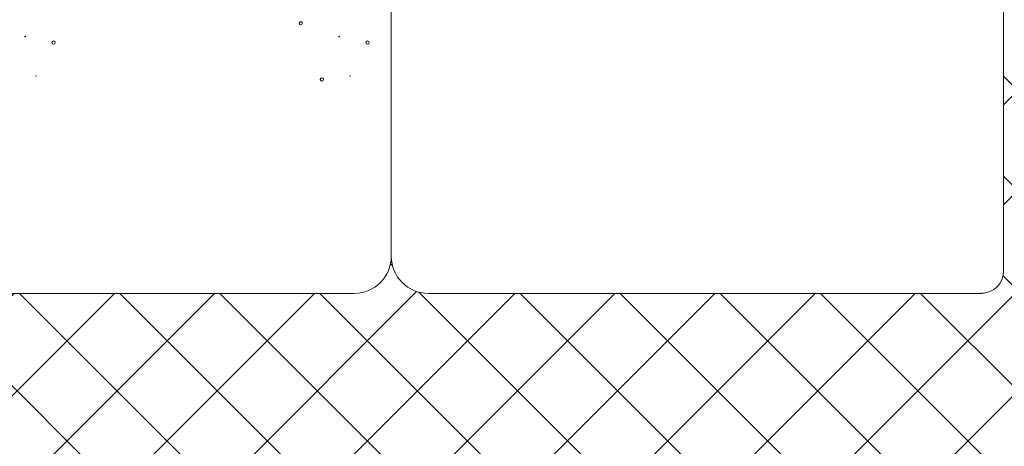
# Model space of a CAD drawing. Units: inches. Extents: x -466983 to 1020, y 324 to 318697.
# Tile 67 of 97: x 644 to 679, y 924 to 939. Entities that reach past the tile are written whole.
import ezdxf

# ---------------------------------------------------------------- set-up
doc = ezdxf.new("R2010")
doc.units = ezdxf.units.IN
doc.header["$MEASUREMENT"] = 0
doc.layers.add('A-FLOR-PATT', color=252, linetype='Continuous', lineweight=13)
doc.layers.add('A-FURN', color=8, linetype='Continuous', lineweight=18)

# ---------------------------------------------------------------- blocks, each defined once
blk = doc.blocks.new('L Shaped Sofa')
at = {"ltscale": 2}
for p, q in [((2356.696, 767.567), (2377.232, 767.567)), ((2377.232, 767.567), (2392.324, 767.567)), ((2429.959, 767.567), (2397.1, 767.567)), ((2355.263, 760.482), (2355.263, 766.134)), ((2394.712, 747.255), (2394.712, 765.179)), ((2355.263, 760.482), (2355.263, 736.259))]:
    blk.add_line(p, q, dxfattribs=at)
for centre, radius, start, end in [((2356.696, 766.134), 1.433, 90, 180), ((2392.324, 765.179), 2.388, 0, 90), ((2397.1, 765.179), 2.388, 90, 180), ((2399.184, 753.788), 0.106, 90, 270), ((2399.184, 753.788), 0.106, 270, 90), ((2397.375, 753.562), 0.0177, 90, 270), ((2397.375, 753.562), 0.0177, 270, 90), ((2417.604, 753.562), 0.0177, 90, 270), ((2417.604, 753.562), 0.0177, 270, 90), ((2396.244, 751.412), 0.106, 90, 270), ((2396.244, 751.412), 0.106, 270, 90), ((2416.474, 751.412), 0.106, 90, 270), ((2416.474, 751.412), 0.106, 270, 90), ((2398.074, 751.018), 0.0177, 90, 270), ((2398.074, 751.018), 0.0177, 270, 90), ((2418.303, 751.018), 0.0177, 90, 270), ((2418.303, 751.018), 0.0177, 270, 90), ((2400.541, 750.168), 0.106, 90, 270), ((2400.541, 750.168), 0.106, 270, 90)]:
    blk.add_arc(centre, radius, start, end, dxfattribs=at)

msp = doc.modelspace()

# ---------------------------------------------------------------- hatches: boundary and pattern name
at = {"layer": 'A-FLOR-PATT', "transparency": 33554572}
h = msp.add_hatch(dxfattribs=at)
h.set_pattern_fill('ANSI37', color=256, scale=30)
h.set_pattern_definition([(45, (-1212.4137, -290.035), (-2.6516504, 2.6516504), []), (135, (-1212.4137, -290.035), (-2.6516504, -2.6516504), [])])
h.paths.add_polyline_path([(901.806, 1075.938), (900.614, 1075.938), (900.614, 1065.386), (899.391, 1065.386), (898.091, 1065.386), (892.836, 1058.71, -0.258377), (892.188, 1058.351), (879.985, 1058.351, -0.20177), (879.438, 1058.581), (874.081, 1065.386), (872.781, 1065.386), (871.558, 1065.386), (871.558, 1075.938), (813.806, 1075.938), (813.806, 1044.792), (832.395, 1044.792, -0.394795), (848.66, 1028.536), (848.66, 1009.938), (901.806, 1009.938), (901.806, 1015.938), (901.306, 1015.938), (871.306, 1015.938), (871.306, 1017.25), (871.334, 1017.25, -0.401453), (901.306, 1045.938), (901.806, 1045.938)])
edge = h.paths.add_edge_path(flags=16)
edge.add_line((847.773, 1068.949), (847.773, 1073.709))
edge.add_arc((849.227, 1073.709), 1.454, 90, 180, ccw=False)
edge.add_line((849.227, 1075.163), (864.492, 1075.163))
edge.add_arc((864.492, 1073.709), 1.454, 0, 90, ccw=False)
edge.add_line((865.946, 1073.709), (865.946, 1069.004))
edge.add_arc((832.645, 1068.976), 33.301, -20.6123, 0.0472, ccw=False)
edge.add_ellipse((856.859, 1058.48), major_axis=(0, 10.213), ratio=0.685919, start_angle=100.0088, end_angle=259.9912, ccw=False)
edge.add_arc((881.074, 1068.976), 33.301, 180.0472, 200.6123, ccw=False)
h.paths.add_polyline_path([(853.146, 1066.482), (853.146, 1066.453), (853.146, 1066.453, 0.433107), (852.917, 1066.685), (852.917, 1066.453), (853.146, 1066.453), (853.146, 1066.482), (853.088, 1066.612, 0.697939), (852.7, 1066.453), (852.7, 1066.453), (852.7, 1066.482), (852.917, 1067.001), (852.917, 1066.685, -0.396254)], flags=0)
h.paths.add_polyline_path([(861.019, 1066.482), (861.019, 1066.453), (861.019, 1066.453, 0.416404), (860.802, 1066.685), (860.802, 1066.453), (861.019, 1066.453), (861.019, 1066.482), (860.967, 1066.605, 0.713344), (860.573, 1066.453), (860.573, 1066.453), (860.573, 1066.482), (860.802, 1067.001), (860.802, 1066.685, -0.379973)], flags=0)
edge = h.paths.add_edge_path(flags=0)
edge.add_spline(control_points=[(861.13, 1065.785), (861.466, 1065.248), (861.613, 1065.016), (861.983, 1064.374), (862.192, 1063.944), (862.561, 1063.039), (862.721, 1062.563), (862.987, 1061.578), (863.092, 1061.069), (863.245, 1060.031), (863.293, 1059.503), (863.329, 1058.441), (863.318, 1057.908), (863.237, 1056.852), (863.166, 1056.329), (862.97, 1055.308), (862.843, 1054.81), (862.537, 1053.852), (862.357, 1053.393), (861.951, 1052.525), (861.725, 1052.117), (861.233, 1051.362), (860.967, 1051.016), (860.405, 1050.395), (860.108, 1050.12), (859.494, 1049.646), (859.176, 1049.448), (858.528, 1049.13), (858.197, 1049.011), (857.531, 1048.852), (857.196, 1048.812), (856.525, 1048.812), (856.189, 1048.852), (855.524, 1049.01), (855.193, 1049.129), (854.545, 1049.447), (854.227, 1049.645), (853.612, 1050.118), (853.316, 1050.393), (852.753, 1051.014), (852.487, 1051.36), (851.995, 1052.114), (851.769, 1052.523), (851.363, 1053.39), (851.183, 1053.85), (850.877, 1054.807), (850.75, 1055.305), (850.553, 1056.326), (850.483, 1056.849), (850.401, 1057.905), (850.39, 1058.438), (850.426, 1059.5), (850.473, 1060.028), (850.626, 1061.066), (850.732, 1061.575), (850.997, 1062.561), (851.157, 1063.036), (851.525, 1063.942), (851.734, 1064.371), (852.106, 1065.016), (852.254, 1065.25), (852.608, 1065.733)], knot_values=[3.915332, 3.915332, 3.915332, 3.915332, 4.013468, 4.013468, 4.175532, 4.175532, 4.337596, 4.337596, 4.49966, 4.49966, 4.661724, 4.661724, 4.823788, 4.823788, 4.985852, 4.985852, 5.147916, 5.147916, 5.30998, 5.30998, 5.472044, 5.472044, 5.634109, 5.634109, 5.796173, 5.796173, 5.958237, 5.958237, 6.120301, 6.120301, 6.282365, 6.282365, 6.444429, 6.444429, 6.606493, 6.606493, 6.768557, 6.768557, 6.930621, 6.930621, 7.092685, 7.092685, 7.254749, 7.254749, 7.416813, 7.416813, 7.578878, 7.578878, 7.740942, 7.740942, 7.903006, 7.903006, 8.06507, 8.06507, 8.227134, 8.227134, 8.389198, 8.389198, 8.551262, 8.551262, 8.65037, 8.65037, 8.65037, 8.65037], degree=3, periodic=0)
edge.add_line((852.642, 1065.785), (861.13, 1065.785))
edge = h.paths.add_edge_path(flags=0)
edge.add_ellipse((856.85, 1057.743), major_axis=(0, 7.792), ratio=0.687861, start_angle=0, end_angle=360)
h.paths.add_polyline_path([(848.863, 1069.389), (848.863, 1073.96, -0.414214), (849.954, 1075.051), (863.765, 1075.051, -0.414214), (864.856, 1073.96), (864.856, 1069.389, -0.388936), (864.524, 1069.027, -0.043561), (849.195, 1069.027, -0.388936)], flags=0)
h.paths.add_polyline_path([(853.101, 1068.112, -1), (852.677, 1068.112, -1)], flags=0)
edge = h.paths.add_edge_path(flags=0)
edge.add_ellipse((856.859, 1057.338), major_axis=(0, 2.207), ratio=0.657164, start_angle=0, end_angle=360)
h.paths.add_polyline_path([(861.041, 1068.112, -1), (860.618, 1068.112, -1)], flags=0)
edge = h.paths.add_edge_path()
edge.add_line((573.954, 1057.341), (573.954, 1075.938))
edge.add_line((573.954, 1075.938), (558.731, 1075.938))
edge.add_line((558.731, 1075.938), (558.731, 1065.386))
edge.add_line((558.731, 1065.386), (557.507, 1065.386))
edge.add_line((557.507, 1065.386), (556.207, 1065.386))
edge.add_line((556.207, 1065.386), (550.952, 1058.71))
edge.add_arc((550.304, 1059.116), 0.765, 270, 327.9483, ccw=False)
edge.add_line((550.304, 1058.351), (538.101, 1058.351))
edge.add_arc((538.101, 1059.116), 0.765, 224.3704, 270, ccw=False)
edge.add_line((537.555, 1058.581), (532.198, 1065.386))
edge.add_line((532.198, 1065.386), (530.898, 1065.386))
edge.add_line((530.898, 1065.386), (529.674, 1065.386))
edge.add_line((529.674, 1065.386), (529.674, 1075.938))
edge.add_line((529.674, 1075.938), (520.806, 1075.938))
edge.add_line((520.806, 1075.938), (520.806, 1045.938))
edge.add_line((520.806, 1045.938), (521.306, 1045.938))
edge.add_arc((521.306, 1015.938), 30, 2.5075, 90, ccw=False)
edge.add_line((551.277, 1017.25), (551.306, 1017.25))
edge.add_line((551.306, 1017.25), (551.306, 1015.938))
edge.add_line((551.306, 1015.938), (520.806, 1015.938))
edge.add_line((520.806, 1015.938), (520.806, 1009.938))
edge.add_line((520.806, 1009.938), (559.191, 1010.402))
edge.add_arc((559.191, 1011.856), 1.454, 180, 270, ccw=False)
edge.add_line((557.737, 1011.856), (557.737, 1016.561))
edge.add_arc((591.039, 1016.589), 33.301, 159.3877, 180.0472, ccw=False)
edge.add_ellipse((566.824, 1027.085), major_axis=(0, 10.213), ratio=0.685919, start_angle=280.0088, end_angle=439.9912, ccw=False)
edge.add_arc((542.609, 1016.589), 33.301, 0.0472, 20.6123, ccw=False)
edge.add_line((575.91, 1016.616), (575.91, 1011.856))
edge.add_arc((574.456, 1011.856), 1.454, -90, 0, ccw=False)
edge.add_line((574.456, 1010.402), (608.806, 1009.938))
edge.add_line((608.806, 1009.938), (608.806, 1041.086))
edge.add_line((608.806, 1041.086), (590.218, 1041.086))
edge.add_arc((590.775, 1057.907), 16.831, 181.9277, 268.1032, ccw=False)
edge = h.paths.add_edge_path()
edge.add_ellipse((494.244, 583.62), major_axis=(0, 10.213), ratio=0.685919, start_angle=280.0088, end_angle=439.9912, ccw=False)
edge.add_arc((470.03, 573.124), 33.301, 0.0472, 20.6123, ccw=False)
edge.add_line((503.331, 573.152), (503.331, 568.392))
edge.add_arc((501.877, 568.392), 1.454, -90, 0, ccw=False)
edge.add_line((501.877, 566.938), (539.806, 566.938))
edge.add_line((539.806, 566.938), (539.806, 572.938))
edge.add_line((539.806, 572.938), (539.306, 572.938))
edge.add_line((539.306, 572.938), (509.306, 572.938))
edge.add_line((509.306, 572.938), (509.306, 574.25))
edge.add_line((509.306, 574.25), (509.334, 574.25))
edge.add_arc((539.306, 572.938), 30, 90, 177.4925, ccw=False)
edge.add_line((539.306, 602.938), (539.806, 602.938))
edge.add_line((539.806, 602.938), (539.806, 626.938))
edge.add_line((539.806, 626.938), (531.772, 626.938))
edge.add_line((531.772, 626.938), (531.772, 616.386))
edge.add_line((531.772, 616.386), (530.548, 616.386))
edge.add_line((530.548, 616.386), (529.249, 616.386))
edge.add_line((529.249, 616.386), (523.711, 609.351))
edge.add_line((523.711, 609.351), (510.777, 609.351))
edge.add_line((510.777, 609.351), (505.239, 616.386))
edge.add_line((505.239, 616.386), (503.939, 616.386))
edge.add_line((503.939, 616.386), (502.715, 616.386))
edge.add_line((502.715, 616.386), (502.715, 626.938))
edge.add_line((502.715, 626.938), (481.698, 626.938))
edge.add_line((481.698, 626.938), (481.698, 610.995))
edge.add_arc((467.27, 611.473), 14.436, 271.9277, 358.1032, ccw=False)
edge.add_line((467.756, 597.045), (451.806, 597.045))
edge.add_line((451.806, 597.045), (451.806, 584.404))
edge.add_line((451.806, 584.404), (451.806, 566.938))
edge.add_line((451.806, 566.938), (486.612, 566.938))
edge.add_arc((486.612, 568.392), 1.454, 180, 270, ccw=False)
edge.add_line((485.158, 568.392), (485.158, 573.097))
edge.add_arc((518.459, 573.124), 33.301, 159.3877, 180.0472, ccw=False)
h.paths.add_polyline_path([(836.261, 1020.733), (879.89, 1020.733), (879.89, 1039.39), (836.261, 1039.39)], flags=25)
h.paths.add_polyline_path([(549.985, 1036.749), (593.614, 1036.749), (593.614, 1055.407), (549.985, 1055.407)], flags=24)
h.paths.add_polyline_path([(475.123, 595.596), (518.752, 595.596), (518.752, 614.253), (475.123, 614.253)], flags=24)
h = msp.add_hatch(dxfattribs=at)
h.set_pattern_fill('ANSI37', color=256, scale=20)
h.set_pattern_definition([(45, (-1212.4137, -290.035), (-1.767767, 1.767767), []), (135, (-1212.4137, -290.035), (-1.767767, -1.767767), [])])
h.paths.add_polyline_path([(809.806, 870.938), (809.806, 888.152), (806.998, 888.152), (802.662, 888.152), (789.383, 888.152), (786.285, 888.152, -0.414214), (785.499, 888.937), (785.499, 900.196), (785.499, 908.47, -0.414214), (786.808, 909.779, -0.414214), (785.499, 911.088), (785.499, 929.101, -0.414214), (786.808, 930.411, -0.414214), (785.499, 931.72), (785.499, 931.904, -0.414214), (784.19, 930.595), (766.722, 930.595, -0.412359), (765.413, 931.896, -0.413741), (764.115, 930.578), (744.578, 930.422, -0.416556), (743.786, 931.207), (743.786, 933.515), (742.215, 933.515), (742.215, 952.024, -0.001344), (743.786, 952.2), (743.786, 953.938), (678.592, 953.938), (678.592, 951.131), (678.592, 946.794), (678.592, 933.515), (678.592, 930.417, -0.414214), (677.806, 929.631), (666.548, 929.631), (658.274, 929.631, -0.414214), (656.965, 930.94, -0.414214), (655.656, 929.631), (637.642, 929.631, -0.414214), (636.333, 930.94, -0.414214), (635.024, 929.631), (634.839, 929.631, -0.414214), (636.149, 928.322), (636.149, 910.854, -0.412359), (634.848, 909.545, -0.413741), (636.165, 908.247), (636.321, 888.71, -0.416556), (635.536, 887.918), (633.228, 887.918), (633.228, 886.347), (614.719, 886.347, -0.001344), (614.544, 887.918), (612.806, 887.918), (612.806, 834.938), (612.806, 752.938), (612.806, 748.938), (612.806, 697.938), (654.806, 697.938), (654.806, 701.938), (715.806, 701.938), (715.806, 737.435), (774.292, 737.435), (774.292, 795.938), (809.806, 795.938)])
h.paths.add_polyline_path([(679.276, 849.576, 0.102523), (682.148, 849.261, -0.080461), (694.543, 849.773, -0.283899), (694.482, 849.008, 0.136605), (694.407, 848.81, -0.030441), (694.543, 846.893), (694.543, 842.62), (694.543, 838.347, -0.028219), (694.425, 836.568), (694.425, 836.568, 0.196187), (694.446, 836.271, -0.302897), (694.543, 835.467, -0.080461), (682.148, 835.979, 0.102523), (679.276, 835.664, -0.58611), (678.646, 836.017), (678.646, 849.223, -0.58611)], flags=16)
h.paths.add_polyline_path([(679.517, 848.651, 0.699597), (679.476, 848.634, 1.20716), (679.194, 848.742, 0.010621)], flags=0)
h.paths.add_polyline_path([(679.492, 836.561, -0.013798), (679.918, 836.659, -0.071703), (682.853, 837.143, -0.165743), (682.166, 839.101), (682.166, 842.609), (682.166, 846.06, -0.240616), (683.473, 848.677, -0.068263), (693.929, 849.008), (693.788, 848.708), (693.788, 849.023, 0.067332), (683.473, 848.677, 0.240616), (682.166, 846.06), (682.166, 842.609), (682.166, 839.101, 0.23459), (683.461, 836.551, 0.068093), (693.788, 836.195), (693.788, 836.51), (693.93, 836.21, -0.077215), (682.242, 836.782, 0.086627), (679.528, 836.57, -0.628402), (679.503, 836.573), (679.503, 836.607, 0.910458)], flags=0)
h.paths.add_polyline_path([(679.476, 848.636), (679.207, 848.647), (679.207, 836.572, 0.913566), (679.365, 836.586), (679.476, 836.582)], flags=0)
h.paths.add_polyline_path([(679.276, 829.86, 0.102523), (682.148, 829.546, -0.080461), (694.543, 830.057, -0.283899), (694.482, 829.293, 0.136605), (694.407, 829.095, -0.030441), (694.543, 827.178), (694.543, 822.904), (694.543, 818.631, -0.028219), (694.425, 816.853), (694.425, 816.853, 0.196187), (694.446, 816.556, -0.302897), (694.543, 815.752, -0.080461), (682.148, 816.263, 0.102523), (679.276, 815.949, -0.58611), (678.646, 816.302), (678.646, 829.507, -0.58611)], flags=16)
h.paths.add_polyline_path([(679.517, 828.936, 0.699597), (679.476, 828.919, 1.20716), (679.194, 829.027, 0.010621)], flags=0)
h.paths.add_polyline_path([(679.492, 816.846, -0.013798), (679.918, 816.944, -0.071703), (682.853, 817.428, -0.165743), (682.166, 819.385), (682.166, 822.894), (682.166, 826.345, -0.240616), (683.473, 828.961, -0.068263), (693.929, 829.293), (693.788, 828.993), (693.788, 829.308, 0.067332), (683.473, 828.961, 0.240616), (682.166, 826.345), (682.166, 822.894), (682.166, 819.385, 0.23459), (683.461, 816.836, 0.068093), (693.788, 816.48), (693.788, 816.795), (693.93, 816.495, -0.077215), (682.242, 817.066, 0.086627), (679.528, 816.855, -0.628402), (679.503, 816.858), (679.503, 816.892, 0.910458)], flags=0)
h.paths.add_polyline_path([(679.476, 828.921), (679.207, 828.932), (679.207, 816.857, 0.913566), (679.365, 816.871), (679.476, 816.867)], flags=0)
h.paths.add_polyline_path([(679.276, 810.145, 0.102523), (682.148, 809.83, -0.080461), (694.543, 810.342, -0.3023), (694.447, 809.539, 0.10023), (694.406, 809.388, -0.03057), (694.543, 807.462), (694.543, 803.189), (694.543, 798.916, -0.03057), (694.406, 796.991, 0.10023), (694.447, 796.839, -0.3023), (694.543, 796.036, -0.080461), (682.148, 796.548, 0.102523), (679.276, 796.233, -0.58611), (678.646, 796.586), (678.646, 809.792, -0.58611)], flags=16)
h.paths.add_polyline_path([(679.517, 809.242, 0.699597), (679.476, 809.224, 1.20716), (679.194, 809.332, 0.010621)], flags=0)
h.paths.add_polyline_path([(679.492, 797.151, -0.013798), (679.918, 797.25, -0.071703), (682.853, 797.734, -0.165743), (682.166, 799.691), (682.166, 803.2), (682.166, 806.65, -0.239349), (683.461, 809.258, -0.072465), (694.447, 809.541, 0.197932), (694.425, 809.241), (693.788, 809.299), (693.788, 809.614, 0.068093), (683.461, 809.258, 0.239349), (682.166, 806.65), (682.166, 803.2), (682.166, 799.691, 0.235854), (683.473, 797.132, 0.067332), (693.788, 796.786), (693.788, 797.101), (694.425, 797.159, 0.197932), (694.447, 796.859, -0.080419), (682.156, 797.379, 0.083867), (679.528, 797.16, -0.628402), (679.503, 797.164), (679.503, 797.197, 0.910458)], flags=0)
h.paths.add_polyline_path([(679.207, 809.237), (679.207, 797.162, 0.913566), (679.365, 797.176), (679.476, 797.173), (679.476, 809.227)], flags=0)
h.paths.add_polyline_path([(695.364, 853.299), (728.223, 853.299), (728.223, 771.152), (695.364, 771.152)], flags=16)
h.paths.add_polyline_path([(696.021, 852.642), (727.566, 852.642), (727.566, 771.809), (696.021, 771.809)], flags=0)
h.paths.add_polyline_path([(679.276, 788.787, 0.102523), (682.148, 788.472, -0.080461), (694.543, 788.984, -0.3023), (694.447, 788.181, 0.10023), (694.406, 788.03, -0.03057), (694.543, 786.104), (694.543, 781.831), (694.543, 777.558, -0.03057), (694.406, 775.632, 0.10023), (694.447, 775.481, -0.3023), (694.543, 774.678, -0.080461), (682.148, 775.19, 0.102523), (679.276, 774.875, -0.58611), (678.646, 775.228), (678.646, 788.434, -0.58611)], flags=16)
h.paths.add_polyline_path([(679.517, 787.883, 0.699597), (679.476, 787.866, 1.20716), (679.194, 787.974, 0.010621)], flags=0)
h.paths.add_polyline_path([(679.492, 775.793, -0.013798), (679.918, 775.891, -0.071703), (682.853, 776.375, -0.165743), (682.166, 778.333), (682.166, 781.841), (682.166, 785.292, -0.239349), (683.461, 787.899, -0.072465), (694.447, 788.182, 0.197932), (694.425, 787.882), (693.788, 787.94), (693.788, 788.255, 0.068093), (683.461, 787.899, 0.239349), (682.166, 785.292), (682.166, 781.841), (682.166, 778.333, 0.235854), (683.473, 775.774, 0.067332), (693.788, 775.428), (693.788, 775.742), (694.425, 775.8, 0.197932), (694.447, 775.5, -0.080419), (682.156, 776.021, 0.083867), (679.528, 775.802, -0.628402), (679.503, 775.805), (679.503, 775.839, 0.910458)], flags=0)
h.paths.add_polyline_path([(679.207, 787.879), (679.207, 775.804, 0.913566), (679.365, 775.818), (679.476, 775.814), (679.476, 787.868)], flags=0)
h.paths.add_polyline_path([(704.641, 854.12, -0.080461), (705.153, 866.516, 0.102523), (704.838, 869.387, -0.58611), (705.191, 870.017), (718.397, 870.017, -0.58611), (718.75, 869.387, 0.102523), (718.435, 866.516, -0.080461), (718.946, 854.12, -0.3023), (718.144, 854.217, 0.10023), (717.992, 854.257, -0.03057), (716.067, 854.12), (711.794, 854.12), (707.521, 854.12, -0.03057), (705.595, 854.257, 0.10023), (705.444, 854.217, -0.3023)], flags=16)
h.paths.add_polyline_path([(717.846, 869.146, 0.699597), (717.829, 869.187, 1.20716), (717.937, 869.47, 0.010621)], flags=0)
h.paths.add_polyline_path([(705.463, 854.216, -0.080419), (705.984, 866.507, 0.083867), (705.765, 869.135, -0.628402), (705.768, 869.16), (705.802, 869.16, 0.910458), (705.756, 869.171, -0.013798), (705.854, 868.745, -0.071703), (706.338, 865.81, -0.165743), (708.295, 866.497), (711.804, 866.497), (715.255, 866.497, -0.239349), (717.862, 865.202, -0.072465), (718.145, 854.216, 0.197932), (717.845, 854.238), (717.903, 854.876), (718.218, 854.876, 0.068093), (717.862, 865.202, 0.239349), (715.255, 866.497), (711.804, 866.497), (708.295, 866.497, 0.235854), (705.737, 865.19, 0.067332), (705.391, 854.876), (705.705, 854.876), (705.763, 854.238, 0.197932)], flags=16)
h.paths.add_polyline_path([(705.766, 869.456, 0.913566), (705.781, 869.299), (705.777, 869.187), (717.831, 869.187), (717.842, 869.456)], flags=0)
h.paths.add_polyline_path([(729.045, 842.62), (729.045, 846.893, -0.03057), (729.182, 848.818, 0.10023), (729.141, 848.97, -0.3023), (729.045, 849.773, -0.080461), (741.44, 849.261, 0.102523), (744.311, 849.576, -0.58611), (744.942, 849.223), (744.942, 836.017, -0.58611), (744.311, 835.664, 0.102523), (741.44, 835.979, -0.080461), (729.045, 835.467, -0.3023), (729.141, 836.27, 0.10023), (729.182, 836.421, -0.03057), (729.045, 838.347)], flags=16)
h.paths.add_polyline_path([(744.111, 836.585, 1.20716), (744.394, 836.477, 0.010621), (744.07, 836.567, 0.699597)], flags=0)
h.paths.add_polyline_path([(729.141, 836.268, 0.197932), (729.162, 836.568), (729.8, 836.51), (729.8, 836.195, 0.068093), (740.126, 836.551, 0.239349), (741.421, 839.159), (741.421, 842.609), (741.421, 846.118, 0.235854), (740.114, 848.677, 0.067332), (729.8, 849.023), (729.8, 848.708), (729.162, 848.65, 0.197932), (729.141, 848.95, -0.080419), (741.432, 848.43, 0.083867), (744.059, 848.649, -0.628402), (744.085, 848.645), (744.085, 848.612, 0.910458), (744.095, 848.658, -0.013798), (743.67, 848.559, -0.071703), (740.734, 848.075, -0.165743), (741.421, 846.118), (741.421, 842.609), (741.421, 839.159, -0.239349), (740.126, 836.551, -0.072465)], flags=0)
h.paths.add_polyline_path([(729.045, 830.057, -0.080461), (741.44, 829.546, 0.102523), (744.311, 829.86, -0.58611), (744.942, 829.507), (744.942, 816.302, -0.58611), (744.311, 815.949, 0.102523), (741.44, 816.263, -0.080461), (729.045, 815.752, -0.3023), (729.141, 816.554, 0.10023), (729.182, 816.706, -0.03057), (729.045, 818.631), (729.045, 822.904), (729.045, 827.178, -0.03057), (729.182, 829.103, 0.10023), (729.141, 829.255, -0.3023)], flags=16)
h.paths.add_polyline_path([(744.111, 816.869, 1.20716), (744.394, 816.761, 0.010621), (744.07, 816.852, 0.699597)], flags=0)
h.paths.add_polyline_path([(729.141, 829.235, -0.080419), (741.432, 828.714, 0.083867), (744.059, 828.933, -0.628402), (744.085, 828.93), (744.085, 828.896, 0.910458), (744.095, 828.943, -0.013798), (743.67, 828.844, -0.071703), (740.734, 828.36, -0.165743), (741.421, 826.403), (741.421, 822.894), (741.421, 819.443, -0.239349), (740.126, 816.836, -0.072465), (729.141, 816.553, 0.197932), (729.162, 816.853), (729.8, 816.795), (729.8, 816.48, 0.068093), (740.126, 816.836, 0.239349), (741.421, 819.443), (741.421, 822.894), (741.421, 826.403, 0.235854), (740.114, 828.961, 0.067332), (729.8, 829.308), (729.8, 828.993), (729.162, 828.935, 0.197932)], flags=16)
h.paths.add_polyline_path([(729.045, 810.342, -0.080461), (741.44, 809.83, 0.102523), (744.311, 810.145, -0.58611), (744.942, 809.792), (744.942, 796.586, -0.58611), (744.311, 796.233, 0.102523), (741.44, 796.548, -0.080461), (729.045, 796.036, -0.283899), (729.105, 796.801, 0.136605), (729.181, 796.999, -0.030441), (729.045, 798.916), (729.045, 803.189), (729.045, 807.462, -0.028219), (729.163, 809.241), (729.162, 809.241, 0.196187), (729.142, 809.538, -0.302897)], flags=16)
h.paths.add_polyline_path([(744.111, 797.175, 1.20716), (744.394, 797.067, 0.010621), (744.07, 797.158, 0.699597)], flags=0)
h.paths.add_polyline_path([(741.345, 809.027, 0.086627), (744.059, 809.239, -0.628402), (744.085, 809.235), (744.085, 809.202, 0.910458), (744.095, 809.248, -0.013798), (743.67, 809.15, -0.071703), (740.734, 808.666, -0.165743), (741.421, 806.708), (741.421, 803.2), (741.421, 799.749, -0.240616), (740.114, 797.132, -0.068263), (729.658, 796.801), (729.8, 797.101), (729.8, 796.786, 0.067332), (740.114, 797.132, 0.240616), (741.421, 799.749), (741.421, 803.2), (741.421, 806.708, 0.23459), (740.126, 809.258, 0.068093), (729.8, 809.614), (729.8, 809.299), (729.658, 809.599, -0.077215)], flags=0)
h.paths.add_polyline_path([(704.641, 770.33, -0.283899), (705.405, 770.27, 0.136605), (705.603, 770.194, -0.030441), (707.521, 770.33), (711.794, 770.33), (716.067, 770.33, -0.028219), (717.845, 770.212), (717.845, 770.213, 0.196187), (718.143, 770.233, -0.302897), (718.946, 770.33, -0.080461), (718.435, 757.935, 0.102523), (718.75, 755.064, -0.58611), (718.397, 754.433), (705.191, 754.433, -0.58611), (704.838, 755.064, 0.102523), (705.153, 757.935, -0.080461)], flags=16)
h.paths.add_polyline_path([(705.762, 755.305, 0.699597), (705.779, 755.264, 1.20716), (705.671, 754.981, 0.010621)], flags=0)
h.paths.add_polyline_path([(705.405, 769.717), (705.705, 769.575), (705.391, 769.575, 0.067332), (705.737, 759.261, 0.240616), (708.353, 757.954), (711.804, 757.954), (715.313, 757.954, 0.23459), (717.862, 759.249, 0.068093), (718.218, 769.575), (717.903, 769.575), (718.203, 769.717, -0.077215), (717.632, 758.03, 0.086627), (717.843, 755.316, -0.628402), (717.84, 755.29), (717.806, 755.29, 0.910458), (717.853, 755.28, -0.013798), (717.754, 755.705, -0.071703), (717.27, 758.641, -0.165743), (715.313, 757.954), (711.804, 757.954), (708.353, 757.954, -0.240616), (705.737, 759.261, -0.068263)], flags=0)
h.paths.add_polyline_path([(729.045, 788.984, -0.080461), (741.44, 788.472, 0.102523), (744.311, 788.787, -0.58611), (744.942, 788.434), (744.942, 775.228, -0.58611), (744.311, 774.875, 0.102523), (741.44, 775.19, -0.080461), (729.045, 774.678, -0.283899), (729.105, 775.443, 0.136605), (729.181, 775.64, -0.030441), (729.045, 777.558), (729.045, 781.831), (729.045, 786.104, -0.028219), (729.163, 787.882), (729.162, 787.882, 0.196187), (729.142, 788.18, -0.302897)], flags=16)
h.paths.add_polyline_path([(744.111, 775.817, 1.20716), (744.394, 775.709, 0.010621), (744.07, 775.799, 0.699597)], flags=0)
h.paths.add_polyline_path([(741.345, 787.669, 0.086627), (744.059, 787.881, -0.628402), (744.085, 787.877), (744.085, 787.844, 0.910458), (744.095, 787.89, -0.013798), (743.67, 787.791, -0.071703), (740.734, 787.307, -0.165743), (741.421, 785.35), (741.421, 781.841), (741.421, 778.39, -0.240616), (740.114, 775.774, -0.068263), (729.658, 775.443), (729.8, 775.742), (729.8, 775.428, 0.067332), (740.114, 775.774, 0.240616), (741.421, 778.39), (741.421, 781.841), (741.421, 785.35, 0.23459), (740.126, 787.899, 0.068093), (729.8, 788.255), (729.8, 787.94), (729.658, 788.241, -0.077215)], flags=0)
h.paths.add_polyline_path([(744.111, 848.636), (744.111, 836.582), (744.381, 836.572), (744.381, 848.647, 0.913566), (744.223, 848.633)], flags=0)
h.paths.add_polyline_path([(744.223, 828.917), (744.111, 828.921), (744.111, 816.867), (744.381, 816.857), (744.381, 828.932, 0.913566)], flags=0)
h.paths.add_polyline_path([(717.831, 755.264), (705.777, 755.264), (705.766, 754.994), (717.842, 754.994, 0.913566), (717.827, 755.152)], flags=0)
h.paths.add_polyline_path([(744.223, 809.223), (744.111, 809.227), (744.111, 797.173), (744.381, 797.162), (744.381, 809.237, 0.913566)], flags=0)
h.paths.add_polyline_path([(744.111, 787.868), (744.111, 775.814), (744.381, 775.804), (744.381, 787.879, 0.913566), (744.223, 787.865)], flags=0)
h.paths.add_polyline_path([(678.877, 877.123), (737.613, 877.123), (737.613, 899.512), (678.877, 899.512)], flags=24)

# ---------------------------------------------------------------- linework, layer by layer
at = {"layer": 'A-FURN', "ltscale": 2}
for p, q in [((678.592, 933.515), (678.592, 946.794)), ((678.592, 933.515), (678.592, 946.794)), ((678.592, 933.515), (678.592, 946.794)), ((678.592, 933.515), (678.592, 946.794)), ((678.592, 933.515), (678.592, 946.794)), ((678.592, 933.515), (678.592, 946.794)), ((656.965, 940.766), (656.965, 930.94)), ((656.965, 940.766), (656.965, 930.94)), ((656.965, 940.766), (656.965, 930.94)), ((656.965, 940.766), (656.965, 930.94)), ((656.965, 940.766), (656.965, 930.94)), ((656.965, 940.766), (656.965, 930.94)), ((678.592, 933.515), (678.592, 930.417)), ((678.592, 933.515), (678.592, 930.417)), ((678.592, 933.515), (678.592, 930.417)), ((678.592, 933.515), (678.592, 930.417)), ((678.592, 933.515), (678.592, 930.417)), ((678.592, 933.515), (678.592, 930.417)), ((637.642, 929.631), (655.656, 929.631)), ((637.642, 929.631), (655.656, 929.631)), ((637.642, 929.631), (655.656, 929.631)), ((637.642, 929.631), (655.656, 929.631)), ((637.642, 929.631), (655.656, 929.631)), ((637.642, 929.631), (655.656, 929.631)), ((666.548, 929.631), (658.274, 929.631)), ((666.548, 929.631), (658.274, 929.631)), ((666.548, 929.631), (658.274, 929.631)), ((666.548, 929.631), (658.274, 929.631)), ((666.548, 929.631), (658.274, 929.631)), ((666.548, 929.631), (658.274, 929.631)), ((677.806, 929.631), (666.548, 929.631)), ((677.806, 929.631), (666.548, 929.631)), ((677.806, 929.631), (666.548, 929.631)), ((677.806, 929.631), (666.548, 929.631)), ((677.806, 929.631), (666.548, 929.631)), ((677.806, 929.631), (666.548, 929.631))]:
    msp.add_line(p, q, dxfattribs=at)
for centre, radius, start, end in [((653.77, 939.17), 0.0582, 90, 270), ((653.77, 939.17), 0.0582, 90, 270), ((653.77, 939.17), 0.0582, 90, 270), ((653.77, 939.17), 0.0582, 90, 270), ((653.77, 939.17), 0.0582, 90, 270), ((653.77, 939.17), 0.0582, 90, 270), ((653.77, 939.17), 0.0582, 270, 90), ((653.77, 939.17), 0.0582, 270, 90), ((653.77, 939.17), 0.0582, 270, 90), ((653.77, 939.17), 0.0582, 270, 90), ((653.77, 939.17), 0.0582, 270, 90), ((653.77, 939.17), 0.0582, 270, 90), ((644.032, 938.704), 0.0097, 90, 270), ((644.032, 938.704), 0.0097, 90, 270), ((644.032, 938.704), 0.0097, 90, 270), ((644.032, 938.704), 0.0097, 90, 270), ((644.032, 938.704), 0.0097, 90, 270), ((644.032, 938.704), 0.0097, 90, 270), ((644.032, 938.704), 0.0097, 270, 90), ((644.032, 938.704), 0.0097, 270, 90), ((644.032, 938.704), 0.0097, 270, 90), ((644.032, 938.704), 0.0097, 270, 90), ((644.032, 938.704), 0.0097, 270, 90), ((644.032, 938.704), 0.0097, 270, 90), ((655.122, 938.704), 0.0097, 90, 270), ((655.122, 938.704), 0.0097, 90, 270), ((655.122, 938.704), 0.0097, 90, 270), ((655.122, 938.704), 0.0097, 90, 270), ((655.122, 938.704), 0.0097, 90, 270), ((655.122, 938.704), 0.0097, 90, 270), ((655.122, 938.704), 0.0097, 270, 90), ((655.122, 938.704), 0.0097, 270, 90), ((655.122, 938.704), 0.0097, 270, 90), ((655.122, 938.704), 0.0097, 270, 90), ((655.122, 938.704), 0.0097, 270, 90), ((655.122, 938.704), 0.0097, 270, 90), ((645.035, 938.487), 0.0582, 90, 270), ((645.035, 938.487), 0.0582, 90, 270), ((645.035, 938.487), 0.0582, 90, 270), ((645.035, 938.487), 0.0582, 90, 270), ((645.035, 938.487), 0.0582, 90, 270), ((645.035, 938.487), 0.0582, 90, 270), ((645.035, 938.487), 0.0582, 270, 90), ((645.035, 938.487), 0.0582, 270, 90), ((645.035, 938.487), 0.0582, 270, 90), ((645.035, 938.487), 0.0582, 270, 90), ((645.035, 938.487), 0.0582, 270, 90), ((645.035, 938.487), 0.0582, 270, 90), ((656.125, 938.487), 0.0582, 90, 270), ((656.125, 938.487), 0.0582, 90, 270), ((656.125, 938.487), 0.0582, 90, 270), ((656.125, 938.487), 0.0582, 90, 270), ((656.125, 938.487), 0.0582, 90, 270), ((656.125, 938.487), 0.0582, 90, 270), ((656.125, 938.487), 0.0582, 270, 90), ((656.125, 938.487), 0.0582, 270, 90), ((656.125, 938.487), 0.0582, 270, 90), ((656.125, 938.487), 0.0582, 270, 90), ((656.125, 938.487), 0.0582, 270, 90), ((656.125, 938.487), 0.0582, 270, 90), ((644.415, 937.309), 0.0097, 90, 270), ((644.415, 937.309), 0.0097, 90, 270), ((644.415, 937.309), 0.0097, 90, 270), ((644.415, 937.309), 0.0097, 90, 270), ((644.415, 937.309), 0.0097, 90, 270), ((644.415, 937.309), 0.0097, 90, 270), ((644.415, 937.309), 0.0097, 270, 90), ((644.415, 937.309), 0.0097, 270, 90), ((644.415, 937.309), 0.0097, 270, 90), ((644.415, 937.309), 0.0097, 270, 90), ((644.415, 937.309), 0.0097, 270, 90), ((644.415, 937.309), 0.0097, 270, 90), ((655.505, 937.309), 0.0097, 90, 270), ((655.505, 937.309), 0.0097, 90, 270), ((655.505, 937.309), 0.0097, 90, 270), ((655.505, 937.309), 0.0097, 90, 270), ((655.505, 937.309), 0.0097, 90, 270), ((655.505, 937.309), 0.0097, 90, 270), ((655.505, 937.309), 0.0097, 270, 90), ((655.505, 937.309), 0.0097, 270, 90), ((655.505, 937.309), 0.0097, 270, 90), ((655.505, 937.309), 0.0097, 270, 90), ((655.505, 937.309), 0.0097, 270, 90), ((655.505, 937.309), 0.0097, 270, 90), ((654.513, 937.185), 0.0582, 90, 270), ((654.513, 937.185), 0.0582, 90, 270), ((654.513, 937.185), 0.0582, 90, 270), ((654.513, 937.185), 0.0582, 90, 270), ((654.513, 937.185), 0.0582, 90, 270), ((654.513, 937.185), 0.0582, 90, 270), ((654.513, 937.185), 0.0582, 270, 90), ((654.513, 937.185), 0.0582, 270, 90), ((654.513, 937.185), 0.0582, 270, 90), ((654.513, 937.185), 0.0582, 270, 90), ((654.513, 937.185), 0.0582, 270, 90), ((654.513, 937.185), 0.0582, 270, 90), ((655.656, 930.94), 1.309, 270, 0), ((655.656, 930.94), 1.309, 270, 0), ((655.656, 930.94), 1.309, 270, 0), ((655.656, 930.94), 1.309, 270, 0), ((655.656, 930.94), 1.309, 270, 0), ((655.656, 930.94), 1.309, 270, 0), ((658.274, 930.94), 1.309, 180, 270), ((658.274, 930.94), 1.309, 180, 270), ((658.274, 930.94), 1.309, 180, 270), ((658.274, 930.94), 1.309, 180, 270), ((658.274, 930.94), 1.309, 180, 270), ((658.274, 930.94), 1.309, 180, 270), ((677.806, 930.417), 0.785, 270, 0), ((677.806, 930.417), 0.785, 270, 0), ((677.806, 930.417), 0.785, 270, 0), ((677.806, 930.417), 0.785, 270, 0), ((677.806, 930.417), 0.785, 270, 0), ((677.806, 930.417), 0.785, 270, 0)]:
    msp.add_arc(centre, radius, start, end, dxfattribs=at)

# ---------------------------------------------------------------- block references
at = {"layer": 'A-FURN', "xscale": 0.5482153745360612, "yscale": 0.5482153745360612, "zscale": 0.5482153745360612, "rotation": 180}
msp.add_blockref('L Shaped Sofa', (1969.783, 1350.423), dxfattribs=at)

doc.saveas('drawing.dxf')
